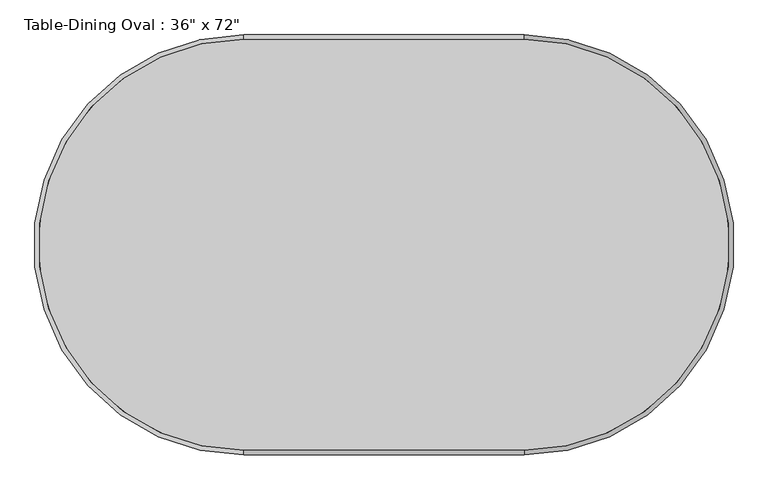
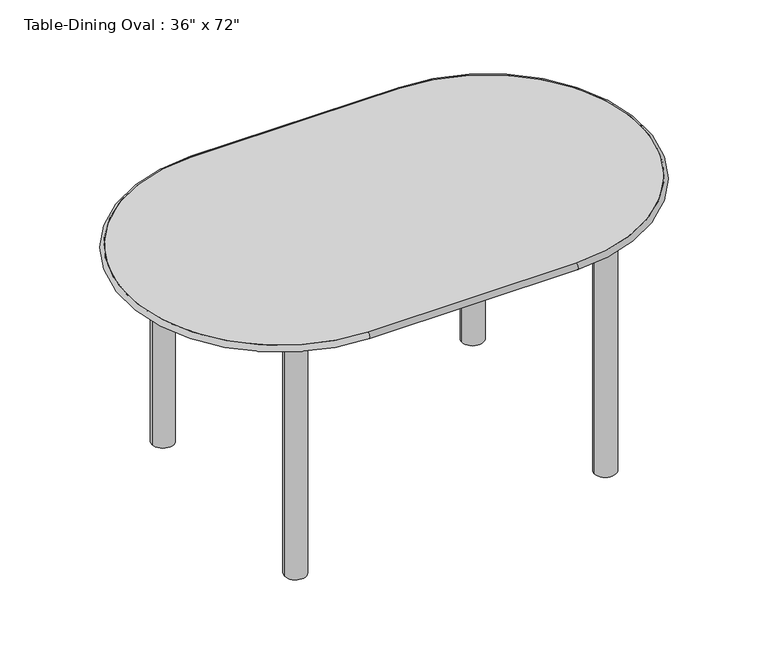
"""IFC4 building model written with IfcOpenShell, lengths in millimetres: furniture geometry."""

from ifc_helpers import new_model, si_unit, point, frame, frame_2d, origin, origin_with_axes, place, context, project, spatial, polyline, circle_curve, ellipse_curve, trimmed, segment, composite_curve, outline, extrude, source, transform, mapped, element, save
from ifc_brep_helpers import plane_surface, cylinder_surface, revolved_surface, advanced_brep


def furniture_582790c0(model_context):
    return source(origin(), model_context, "Body", "SolidModel", [
        advanced_brep(
        [(-706.6196721, -805.7733607, 762.0), (-706.6196721, -805.7733607, 742.95), (-97.0196721, -805.7733607, 742.95), (-97.0196721, -805.7733607, 762.0), (-97.0196721, 89.5766393, 762.0), (-97.0196721, 89.5766393, 742.95), (-706.6196721, 89.5766393, 742.95), (-706.6196721, 89.5766393, 762.0)],
        [
            (0, 1, circle_curve(frame((-706.6196721, -805.7733607, 752.475), z_axis=(1.0, 0.0, 0.0), x_axis=(0.0, 1.0, 0.0)), 9.525)),
            (1, 2),
            (2, 3, circle_curve(frame((-97.0196721, -805.7733607, 752.475), z_axis=(-1.0, 0.0, 0.0), x_axis=(0.0, 1.0, 0.0)), 9.525)),
            (3, 0),
            (1, 0),
            (3, 2),
            (4, 3, circle_curve(frame((-97.0196721, -358.0983607, 762.0), z_axis=(0.0, 0.0, -1.0), x_axis=(0.0, -1.0, 0.0)), 447.675)),
            (2, 5, circle_curve(frame((-97.0196721, -358.0983607, 742.95), z_axis=(0.0, 0.0, 1.0), x_axis=(0.0, -1.0, 0.0)), 447.675)),
            (5, 4, circle_curve(frame((-97.0196721, 89.5766393, 752.475), z_axis=(1.0, 0.0, 0.0), x_axis=(0.0, -1.0, 0.0)), 9.525)),
            (4, 5),
            (5, 6),
            (6, 7, circle_curve(frame((-706.6196721, 89.5766393, 752.475), z_axis=(1.0, 0.0, 0.0), x_axis=(0.0, -1.0, 0.0)), 9.525)),
            (7, 4),
            (7, 6),
            (0, 7, circle_curve(frame((-706.6196721, -358.0983607, 762.0), z_axis=(0.0, 0.0, -1.0), x_axis=(0.0, 1.0, 0.0)), 447.675)),
            (6, 1, circle_curve(frame((-706.6196721, -358.0983607, 742.95), z_axis=(0.0, 0.0, 1.0), x_axis=(0.0, 1.0, 0.0)), 447.675)),
        ],
        [
            cylinder_surface(frame((-706.6196721, -805.7733607, 752.475), z_axis=(-1.0, 0.0, 0.0), x_axis=(0.0, 1.0, 0.0)), 9.525),
            plane_surface(frame((-706.6196721, -805.7733607, 762.0), z_axis=(0.0, 1.0, 0.0), x_axis=(1.0, 0.0, 0.0))),
            revolved_surface(trimmed(ellipse_curve(frame((-97.0196721, -805.7733607, 752.475), z_axis=(-1.0, 0.0, 0.0), x_axis=(0.0, 1.0, 0.0)), 9.525, 9.525), [point((-97.0196721, -805.7733607, 742.95))], [point((-97.0196721, -805.7733607, 762.0))], True, "CARTESIAN"), (-97.0196721, -358.0983607, 0.0), (0.0, 0.0, 1.0)),
            revolved_surface(polyline([(-97.0196721, -805.7733607, 762.0), (-97.0196721, -805.7733607, 742.95)]), (-97.0196721, -358.0983607, 0.0), (0.0, 0.0, 1.0)),
            cylinder_surface(frame((-97.0196721, 89.5766393, 752.475), z_axis=(1.0, 0.0, 0.0), x_axis=(0.0, -1.0, 0.0)), 9.525),
            plane_surface(frame((-97.0196721, 89.5766393, 762.0), z_axis=(0.0, -1.0, 0.0), x_axis=(-1.0, 0.0, 0.0))),
            revolved_surface(trimmed(ellipse_curve(frame((-706.6196721, 89.5766393, 752.475), z_axis=(1.0, 0.0, 0.0), x_axis=(0.0, -1.0, 0.0)), 9.525, 9.525), [point((-706.6196721, 89.5766393, 742.95))], [point((-706.6196721, 89.5766393, 762.0))], True, "CARTESIAN"), (-706.6196721, -358.0983607, 0.0), (0.0, 0.0, 1.0)),
            revolved_surface(polyline([(-706.6196721, 89.57663930000001, 762.0), (-706.6196721, 89.57663930000001, 742.95)]), (-706.6196721, -358.0983607, 0.0), (0.0, 0.0, 1.0)),
        ],
        [
            (0, [[1, 2, 3, 4]]),
            (1, [[5, -4, 6, -2]]),
            (2, [[7, -3, 8, 9]]),
            (3, [[-8, -6, -7, 10]]),
            (4, [[-9, 11, 12, 13]]),
            (5, [[-10, -13, 14, -11]]),
            (6, [[15, -12, 16, -1]]),
            (7, [[-16, -14, -15, -5]]),
        ],
    ),
        extrude(outline(composite_curve([segment(trimmed(circle_curve(frame_2d((-855.8446721, -21.5483607)), 31.75), [point((-887.5946721, -21.5483607))], [point((-824.0946721, -21.5483607))], False, "CARTESIAN"), True, "CONTINUOUS"), segment(trimmed(circle_curve(frame_2d((-855.8446721, -21.5483607)), 31.75), [point((-824.0946721, -21.5483607))], [point((-887.5946721, -21.5483607))], False, "CARTESIAN"), True, "CONTINUOUS")], self_intersect=False)), origin_with_axes(), (0.0, 0.0, 1.0), 742.95),
        extrude(outline(composite_curve([segment(trimmed(circle_curve(frame_2d((-855.8446721, -694.6483607)), 31.75), [point((-887.5946721, -694.6483607))], [point((-824.0946721, -694.6483607))], False, "CARTESIAN"), True, "CONTINUOUS"), segment(trimmed(circle_curve(frame_2d((-855.8446721, -694.6483607)), 31.75), [point((-824.0946721, -694.6483607))], [point((-887.5946721, -694.6483607))], False, "CARTESIAN"), True, "CONTINUOUS")], self_intersect=False)), origin_with_axes(), (0.0, 0.0, 1.0), 742.95),
        extrude(outline(composite_curve([segment(trimmed(circle_curve(frame_2d((52.2053279, -21.5483607)), 31.75), [point((20.4553279, -21.5483607))], [point((83.9553279, -21.5483607))], False, "CARTESIAN"), True, "CONTINUOUS"), segment(trimmed(circle_curve(frame_2d((52.2053279, -21.5483607)), 31.75), [point((83.9553279, -21.5483607))], [point((20.4553279, -21.5483607))], False, "CARTESIAN"), True, "CONTINUOUS")], self_intersect=False)), origin_with_axes(), (0.0, 0.0, 1.0), 742.95),
        extrude(outline(composite_curve([segment(trimmed(circle_curve(frame_2d((52.2053279, -694.6483607)), 31.75), [point((20.4553279, -694.6483607))], [point((83.9553279, -694.6483607))], False, "CARTESIAN"), True, "CONTINUOUS"), segment(trimmed(circle_curve(frame_2d((52.2053279, -694.6483607)), 31.75), [point((83.9553279, -694.6483607))], [point((20.4553279, -694.6483607))], False, "CARTESIAN"), True, "CONTINUOUS")], self_intersect=False)), origin_with_axes(), (0.0, 0.0, 1.0), 742.95),
        extrude(outline(polyline([(71.2553279, -2.4983607), (71.2553279, -713.6983607), (-874.8946721, -713.6983607), (-874.8946721, -2.4983607), (71.2553279, -2.4983607)]), holes=[polyline([(52.2053279, -21.5483607), (-855.8446721, -21.5483607), (-855.8446721, -694.6483607), (52.2053279, -694.6483607), (52.2053279, -21.5483607)])]), frame((0.0, 0.0, 692.15), z_axis=(0.0, 0.0, 1.0), x_axis=(1.0, 0.0, 0.0)), (0.0, 0.0, 1.0), 50.8),
        extrude(outline(composite_curve([segment(polyline([(-706.6196721, 89.5766393), (-97.0196721, 89.5766393)]), True, "CONTINUOUS"), segment(trimmed(circle_curve(frame_2d((-97.0196721, -358.0983607)), 447.675), [point((-97.0196721, 89.5766393))], [point((350.6553279, -358.0983607))], False, "CARTESIAN"), True, "CONTINUOUS"), segment(trimmed(circle_curve(frame_2d((-97.0196721, -358.0983607)), 447.675), [point((350.6553279, -358.0983607))], [point((-97.0196721, -805.7733607))], False, "CARTESIAN"), True, "CONTINUOUS"), segment(polyline([(-97.0196721, -805.7733607), (-706.6196721, -805.7733607)]), True, "CONTINUOUS"), segment(trimmed(circle_curve(frame_2d((-706.6196721, -358.0983607)), 447.675), [point((-706.6196721, -805.7733607))], [point((-1154.2946721, -358.0983607))], False, "CARTESIAN"), True, "CONTINUOUS"), segment(trimmed(circle_curve(frame_2d((-706.6196721, -358.0983607)), 447.675), [point((-1154.2946721, -358.0983607))], [point((-706.6196721, 89.5766393))], False, "CARTESIAN"), True, "CONTINUOUS")], self_intersect=False)), frame((0.0, 0.0, 742.95), z_axis=(0.0, 0.0, 1.0), x_axis=(1.0, 0.0, 0.0)), (0.0, 0.0, 1.0), 19.05),
    ])


if __name__ == "__main__":
    model = new_model("IFC4")
    model_context = context("Model", 3, world=origin())
    ifc_project = project(units=[si_unit("LENGTHUNIT", "METRE", prefix="MILLI")], contexts=[model_context])
    site = spatial("IfcSite", under=ifc_project)
    building = spatial("IfcBuilding", under=site)
    placement = place(None, origin())
    furniture_shape = furniture_582790c0(model_context)
    element("IfcFurniture", 1, ObjectType="Table-Dining Oval : 36\" x 72\"", at=placement, inside=building, context=model_context, shape_type="MappedRepresentation", body=[
        mapped(furniture_shape, transform((0.0, 0.0, 0.0), x_axis=(1.0, 0.0, 0.0), y_axis=(0.0, 1.0, 0.0), z_axis=(0.0, 0.0, 1.0))),
    ])
    save(model, "model.ifc")

# Revit data of these elements
# Type "Table-Dining Oval : 36\" x 72\""
#   Assembly Code = "E2020200"
#   Length = 5' - 0"
#   Width = 3' - 0"
#   Base Material = Steel, Chrome Plated
#   Top Material = Glass - Clear, Grey
#   Default Elevation = 0
#   Description = (empty or 0)
# Element 1 (IfcFurniture, "Table-Dining Oval : 36\" x 72\"")
#   Materials on its faces: "Steel, Chrome Plated", "Glass - Clear, Grey"
# Materials
#   "Steel, Chrome Plated": class "Metal", colour RGB 17 17 17, transparency 0, Description = "Chromiuim plated steel", Cost = 0
#   "Glass - Clear, Grey": class "Glass", colour RGB 252 255 255, transparency 0.64
